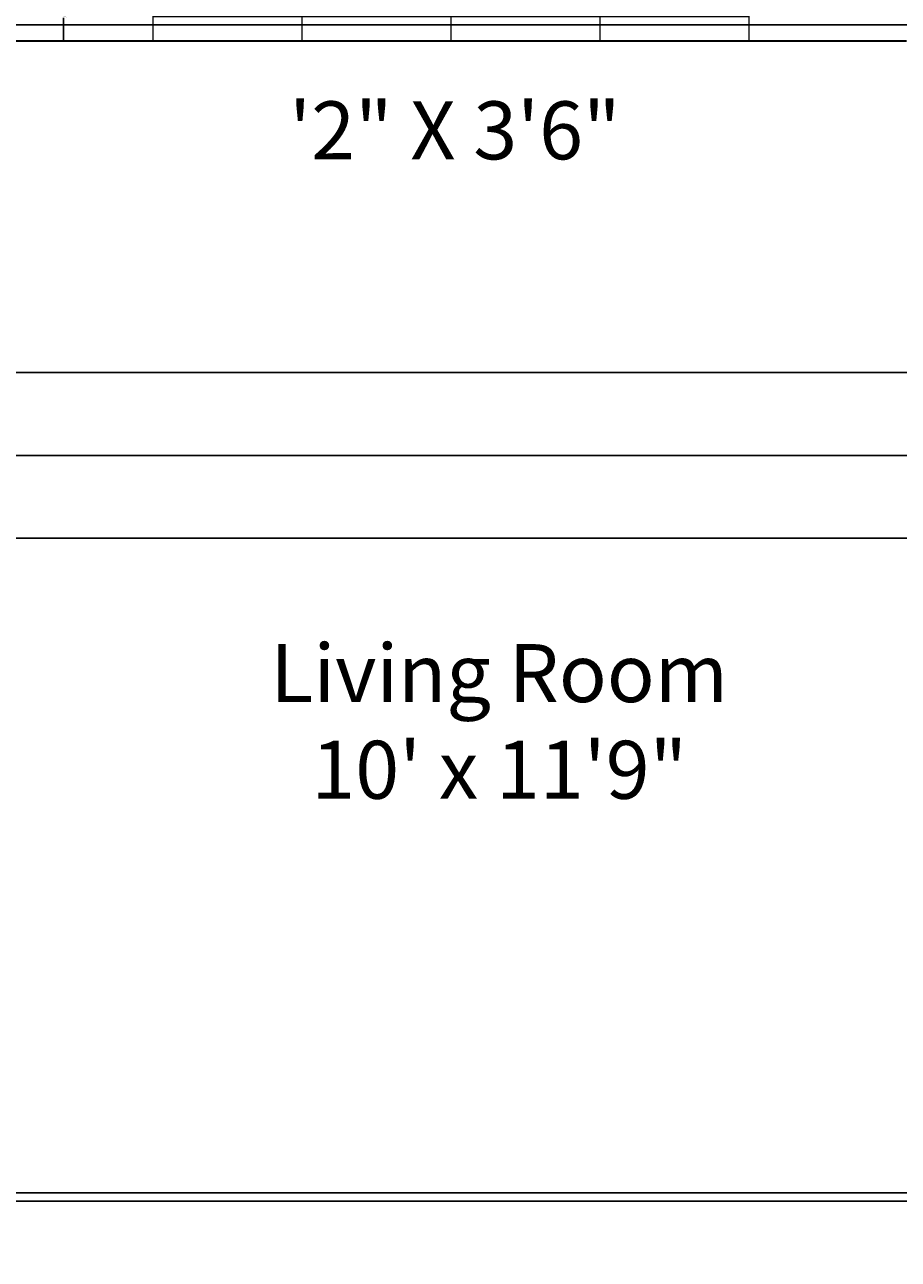
# Model space of a CAD drawing. Units: feet. Extents: x 105 to 1094, y -88 to 588.
# Tile 45 of 59: x 656 to 762, y 288 to 437. Entities that reach past the tile are written whole.
import ezdxf

# ---------------------------------------------------------------- set-up
doc = ezdxf.new("R2010")
doc.units = ezdxf.units.FT
doc.header["$MEASUREMENT"] = 0
for name, color, linetype, lineweight in [('A-ANNO-DIMS', 2, 'Continuous', 18), ('A-AREA-IDEN', 7, 'Continuous', 18), ('A-GLAZ', 4, 'Continuous', 18), ('A-WALL', 7, 'Continuous', 35)]:
    doc.layers.add(name, color=color, linetype=linetype, lineweight=lineweight)
doc.styles.get("Standard").update_dxf_attribs({"font": 'arial.ttf'})
doc.dimstyles.get("Standard").update_dxf_attribs({"dimtxt": 0.18, "dimasz": 0.18, "dimexe": 0.18, "dimexo": 0.0625, "dimgap": 0.09, "dimtad": 0, "dimtih": 1, "dimtoh": 1, "dimdec": 4, "dimzin": 0, "dimdsep": 46, "dimtxsty": 'Standard', "dimcen": 0.09, "dimadec": 0, "dimazin": 0, "dimtfac": 1, "dimtdec": 4, "dimtofl": 0, "dimtmove": 0, "dimatfit": 3, "dimfxl": 1, "dimtolj": 1, "dimtzin": 0, "dimarcsym": 0})

# ---------------------------------------------------------------- blocks, each defined once
blk = doc.blocks.new('WIN-FOUR-LIGHT-WIDE')
for p, q in [((0, 0), (0, 6)), ((18, 0), (18, 6)), ((36, 0), (36, 6)), ((54, 0), (54, 6)), ((72, 0), (72, 6)), ((0, 3), (72, 3)), ((18, 4), (36, 4)), ((54, 4), (72, 4)), ((0, 2), (18, 2)), ((36, 2), (54, 2))]:
    blk.add_line(p, q)
blk = doc.blocks.new('*D13')
at = {"layer": 'A-ANNO-DIMS', "color": 0, "lineweight": -2, "transparency": 16777216}
for p, q in [((671.63, 441.08), (660.71, 441.08)), ((660.89, 440.9), (660.89, 438.26)), ((660.89, 435.26), (660.89, 437.9)), ((671.63, 435.08), (660.71, 435.08))]:
    blk.add_line(p, q, dxfattribs=at)
at = {"layer": 'A-ANNO-DIMS', "color": 0, "transparency": 16777216}
for points in [[(660.86, 440.9), (660.92, 440.9), (660.89, 441.08)], [(660.86, 435.26), (660.92, 435.26), (660.89, 435.08)]]:
    blk.add_solid(points, dxfattribs=at)
at = {"layer": 'Defpoints', "color": 0, "transparency": 16777216}
for p in [(660.89, 441.08), (671.69, 441.08), (671.69, 435.08)]:
    blk.add_point(p, dxfattribs=at)
at = {"layer": 'A-ANNO-DIMS', "color": 0, "transparency": 16777216, "insert": (660.89, 438.08), "char_height": 0.18, "attachment_point": 5}
blk.add_mtext('\\A1;6 TYP.', dxfattribs=at)
blk = doc.blocks.new('*D21')
at = {"layer": 'A-ANNO-DIMS', "color": 0, "lineweight": -2, "transparency": 16777216}
for p, q in [((849.63, 543.08), (105.46, 543.08)), ((105.64, 542.9), (105.64, 250.26)), ((105.64, -42.74), (105.64, 249.9)), ((849.63, -42.92), (105.46, -42.92))]:
    blk.add_line(p, q, dxfattribs=at)
at = {"layer": 'A-ANNO-DIMS', "color": 0, "transparency": 16777216}
for points in [[(105.61, 542.9), (105.67, 542.9), (105.64, 543.08)], [(105.61, -42.74), (105.67, -42.74), (105.64, -42.92)]]:
    blk.add_solid(points, dxfattribs=at)
at = {"layer": 'Defpoints', "color": 0, "transparency": 16777216}
for p in [(105.64, 543.08), (849.69, 543.08), (849.69, -42.92)]:
    blk.add_point(p, dxfattribs=at)
at = {"layer": 'A-ANNO-DIMS', "color": 0, "transparency": 16777216, "insert": (105.64, 250.08), "char_height": 0.18, "attachment_point": 5}
blk.add_mtext('\\A1;586', dxfattribs=at)
blk = doc.blocks.new('*D34')
at = {"layer": 'A-ANNO-DIMS', "color": 0, "lineweight": -2, "transparency": 16777216}
for p, q in [((552.75, 295.08), (1093.92, 295.08)), ((1093.74, 294.9), (1093.74, 253.76)), ((1093.74, 212.26), (1093.74, 253.4)), ((552.75, 212.08), (1093.92, 212.08))]:
    blk.add_line(p, q, dxfattribs=at)
at = {"layer": 'A-ANNO-DIMS', "color": 0, "transparency": 16777216}
for points in [[(1093.71, 294.9), (1093.77, 294.9), (1093.74, 295.08)], [(1093.71, 212.26), (1093.77, 212.26), (1093.74, 212.08)]]:
    blk.add_solid(points, dxfattribs=at)
at = {"layer": 'Defpoints', "color": 0, "transparency": 16777216}
for p in [(552.69, 295.08), (552.69, 212.08), (1093.74, 212.08)]:
    blk.add_point(p, dxfattribs=at)
at = {"layer": 'A-ANNO-DIMS', "color": 0, "transparency": 16777216, "insert": (1093.74, 253.58), "char_height": 0.18, "attachment_point": 5}
blk.add_mtext('\\A1;83', dxfattribs=at)
blk = doc.blocks.new('*D45')
at = {"layer": 'A-ANNO-DIMS', "color": 0, "lineweight": -2, "transparency": 16777216}
for p, q in [((552.75, 437.08), (1093.92, 437.08)), ((1093.74, 436.9), (1093.74, 416.26)), ((1093.74, 395.26), (1093.74, 415.9)), ((552.75, 395.08), (1093.92, 395.08))]:
    blk.add_line(p, q, dxfattribs=at)
at = {"layer": 'A-ANNO-DIMS', "color": 0, "transparency": 16777216}
for points in [[(1093.71, 436.9), (1093.77, 436.9), (1093.74, 437.08)], [(1093.71, 395.26), (1093.77, 395.26), (1093.74, 395.08)]]:
    blk.add_solid(points, dxfattribs=at)
at = {"layer": 'Defpoints', "color": 0, "transparency": 16777216}
for p in [(552.69, 437.08), (552.69, 395.08), (1093.74, 395.08)]:
    blk.add_point(p, dxfattribs=at)
at = {"layer": 'A-ANNO-DIMS', "color": 0, "transparency": 16777216, "insert": (1093.74, 416.08), "char_height": 0.18, "attachment_point": 5}
blk.add_mtext('\\A1;42', dxfattribs=at)
blk = doc.blocks.new('*D50')
at = {"layer": 'A-ANNO-DIMS', "color": 0, "lineweight": -2, "transparency": 16777216}
for p, q in [((552.75, 385.08), (1093.92, 385.08)), ((1093.74, 384.9), (1093.74, 380.26)), ((1093.74, 375.26), (1093.74, 379.9)), ((552.75, 375.08), (1093.92, 375.08))]:
    blk.add_line(p, q, dxfattribs=at)
at = {"layer": 'A-ANNO-DIMS', "color": 0, "transparency": 16777216}
for points in [[(1093.71, 384.9), (1093.77, 384.9), (1093.74, 385.08)], [(1093.71, 375.26), (1093.77, 375.26), (1093.74, 375.08)]]:
    blk.add_solid(points, dxfattribs=at)
at = {"layer": 'Defpoints', "color": 0, "transparency": 16777216}
for p in [(552.69, 385.08), (552.69, 375.08), (1093.74, 375.08)]:
    blk.add_point(p, dxfattribs=at)
at = {"layer": 'A-ANNO-DIMS', "color": 0, "transparency": 16777216, "insert": (1093.74, 380.08), "char_height": 0.18, "attachment_point": 5}
blk.add_mtext('\\A1;10', dxfattribs=at)
blk = doc.blocks.new('*D54')
at = {"layer": 'A-ANNO-DIMS', "color": 0, "lineweight": -2, "transparency": 16777216}
for p, q in [((294.75, 296.08), (1093.92, 296.08)), ((1093.74, 295.9), (1093.74, 286.26)), ((1093.74, 276.26), (1093.74, 285.9)), ((294.75, 276.08), (1093.92, 276.08))]:
    blk.add_line(p, q, dxfattribs=at)
at = {"layer": 'A-ANNO-DIMS', "color": 0, "transparency": 16777216}
for points in [[(1093.71, 295.9), (1093.77, 295.9), (1093.74, 296.08)], [(1093.71, 276.26), (1093.77, 276.26), (1093.74, 276.08)]]:
    blk.add_solid(points, dxfattribs=at)
at = {"layer": 'Defpoints', "color": 0, "transparency": 16777216}
for p in [(294.69, 296.08), (1093.74, 296.08), (294.69, 276.08)]:
    blk.add_point(p, dxfattribs=at)
at = {"layer": 'A-ANNO-DIMS', "color": 0, "transparency": 16777216, "insert": (1093.74, 286.08), "char_height": 0.18, "attachment_point": 5}
blk.add_mtext('\\A1;20', dxfattribs=at)

msp = doc.modelspace()

# ---------------------------------------------------------------- linework, layer by layer
at = {"layer": 'A-WALL'}
msp.add_line((762.6883, 435.0812), (652.6883, 435.0812), dxfattribs=at)

# ---------------------------------------------------------------- block references
at = {"layer": 'A-GLAZ'}
msp.add_blockref('WIN-FOUR-LIGHT-WIDE', (671.688, 435.081), dxfattribs=at)

# ---------------------------------------------------------------- texts
at = {"layer": 'A-ANNO-DIMS', "insert": (658.9665, 427.8248), "char_height": 7, "attachment_point": 1}
msp.add_mtext_dynamic_manual_height_columns('\\pxqc;\'2" X 3\'6"', width=98.34246, gutter_width=1, heights=[0], dxfattribs=at)
at = {"layer": 'A-AREA-IDEN', "insert": (664.3247, 362.3098), "char_height": 7, "attachment_point": 1}
msp.add_mtext_dynamic_manual_height_columns('\\pxqc;Living Room \\P10\' x 11\'9"', width=98.34246, gutter_width=1, heights=[0], dxfattribs=at)

# ---------------------------------------------------------------- dimensions: what is measured, and where the dimension line sits
at = {"layer": 'A-ANNO-DIMS'}
for base, p1, p2, picture, middle in [((105.6383, 543.0812), (849.6883, -42.9188), (849.6883, 543.0812), '*D21', (105.6383, 250.0812)), ((1093.7383, 395.0812), (552.6883, 437.0812), (552.6883, 395.0812), '*D45', (1093.7383, 416.0812)), ((1093.7383, 375.0812), (552.6883, 385.0812), (552.6883, 375.0812), '*D50', (1093.7383, 380.0812)), ((1093.7383, 296.0812), (294.6883, 276.0812), (294.6883, 296.0812), '*D54', (1093.7383, 286.0812)), ((1093.7383, 212.0812), (552.6883, 295.0812), (552.6883, 212.0812), '*D34', (1093.7383, 253.5812))]:
    dim = msp.add_linear_dim(base=base, p1=p1, p2=p2, angle=90, dimstyle='Standard', override={"dimdec": 0, "dimlfac": 1, "dimrnd": 0, "dimzin": 0, "dimdsep": 46, "dimlunit": 2}, dxfattribs=at)
    dim.commit()
    dim.dimension.update_dxf_attribs({"geometry": picture, "text_midpoint": middle})
dim = msp.add_linear_dim(base=(660.8883, 441.0812), p1=(671.6883, 435.0812), p2=(671.6883, 441.0812), angle=90, text='<> TYP.', dimstyle='Standard', override={"dimdec": 0, "dimlfac": 1, "dimrnd": 0, "dimzin": 0, "dimdsep": 46, "dimlunit": 2}, dxfattribs=at)
dim.commit()
dim.dimension.update_dxf_attribs({"geometry": '*D13', "text_midpoint": (660.8883, 438.0812)})

doc.saveas('drawing.dxf')
